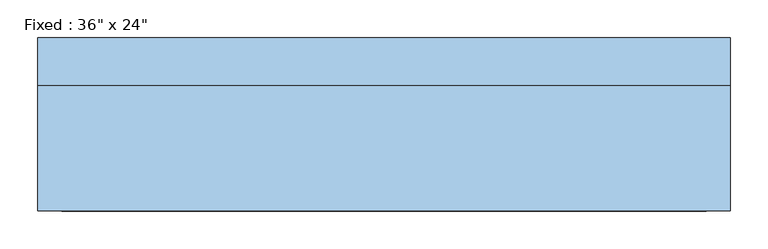
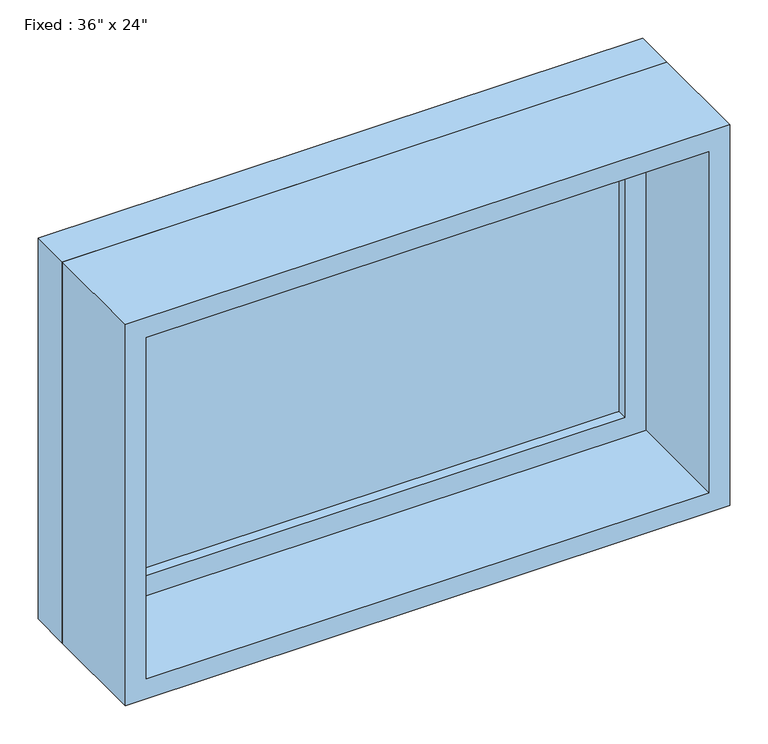
"""IFC4 building model written with IfcOpenShell, lengths in millimetres: window geometry."""

from ifc_helpers import new_model, si_unit, frame, origin, place, context, project, spatial, polyline, outline, extrude, source, transform, mapped, element, save


def window_a7c9e031(model_context):
    return source(origin(), model_context, "Body", "SweptSolid", [
        extrude(outline(polyline([(355.6, 66.675), (-431.8, 66.675), (-431.8, 79.375), (355.6, 79.375), (355.6, 66.675)])), frame((0.0, 0.0, 2197.1), z_axis=(0.0, 0.0, 1.0), x_axis=(1.0, 0.0, 0.0)), (0.0, 0.0, 1.0), 482.6),
        extrude(outline(polyline([(2724.15, -476.25), (2152.65, -476.25), (2152.65, 400.05), (2724.15, 400.05), (2724.15, -476.25)]), holes=[polyline([(2679.7, -431.8), (2679.7, 355.6), (2197.1, 355.6), (2197.1, -431.8), (2679.7, -431.8)])]), frame((0.0, 50.8, 0.0), z_axis=(0.0, 1.0, 0.0), x_axis=(0.0, 0.0, 1.0)), (0.0, 0.0, 1.0), 44.45),
        extrude(outline(polyline([(2743.2, -495.3), (2133.6, -495.3), (2133.6, 419.1), (2743.2, 419.1), (2743.2, -495.3)]), holes=[polyline([(2711.45, -463.55), (2711.45, 387.35), (2165.35, 387.35), (2165.35, -463.55), (2711.45, -463.55)])]), frame((0.0, -114.3, 0.0), z_axis=(0.0, 1.0, 0.0), x_axis=(0.0, 0.0, 1.0)), (0.0, 0.0, 1.0), 165.1),
        extrude(outline(polyline([(2743.2, 419.1), (2743.2, -495.3), (2133.6, -495.3), (2133.6, 419.1), (2743.2, 419.1)]), holes=[polyline([(2724.15, 400.05), (2152.65, 400.05), (2152.65, -476.25), (2724.15, -476.25), (2724.15, 400.05)])]), frame((0.0, 50.8, 0.0), z_axis=(0.0, 1.0, 0.0), x_axis=(0.0, 0.0, 1.0)), (0.0, 0.0, 1.0), 63.5),
    ])


if __name__ == "__main__":
    model = new_model("IFC4")
    model_context = context("Model", 3, world=origin())
    ifc_project = project(units=[si_unit("LENGTHUNIT", "METRE", prefix="MILLI")], contexts=[model_context])
    site = spatial("IfcSite", under=ifc_project)
    building = spatial("IfcBuilding", under=site)
    placement = place(None, origin())
    window_shape = window_a7c9e031(model_context)
    element("IfcWindow", 1, ObjectType="Fixed : 36\" x 24\"", at=placement, inside=building, context=model_context, shape_type="MappedRepresentation", body=[
        mapped(window_shape, transform((0.0, 0.0, 0.0), x_axis=(1.0, 0.0, 0.0), y_axis=(0.0, 1.0, 0.0), z_axis=(0.0, 0.0, 1.0))),
    ])
    save(model, "model.ifc")

# Revit data of these elements
# Type "Fixed : 36\" x 24\""
#   Type Mark = "8"
#   Construction Type Id = "GSP4R"
#   Assembly Code = "B2020100"
#   Analytic Construction = "1/8 in Pilkington single glazing"
#   Visual Light Transmittance = 0.9
#   Solar Heat Gain Coefficient = 0.78
#   Heat Transfer Coefficient (U) = 0.6496 BTU/(h·ft²·°F)
#   Height = 2' - 0"
#   Default Sill Height = 7' - 0"
#   Width = 3' - 0"
#   Window Inset = 0' - 0 3/4"
#   Define Thermal Properties by = 1
#   Define Thermal Properties by = 1
#   Glass Pane Material = Glass
#   Sash Material = Sash
#   Wall Closure = (empty or 0)
# Element 1 (IfcWindow, "Fixed : 36\" x 24\"")
#   Materials on its faces: "Sash", "Glass"
# Materials
#   "Glass": class "Glass", colour RGB 0 128 192, transparency 0.75, Description = "Soda Lime Glass", Cost = 0
#   "Sash": class "Wood", colour RGB 224 178 126, transparency 0, Cost = 0
